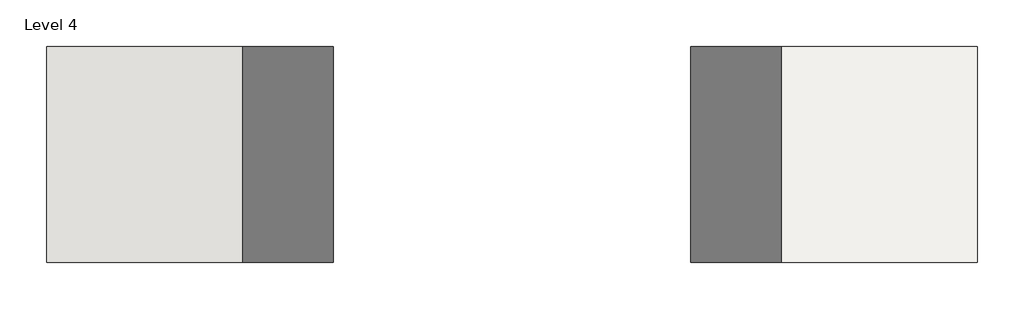
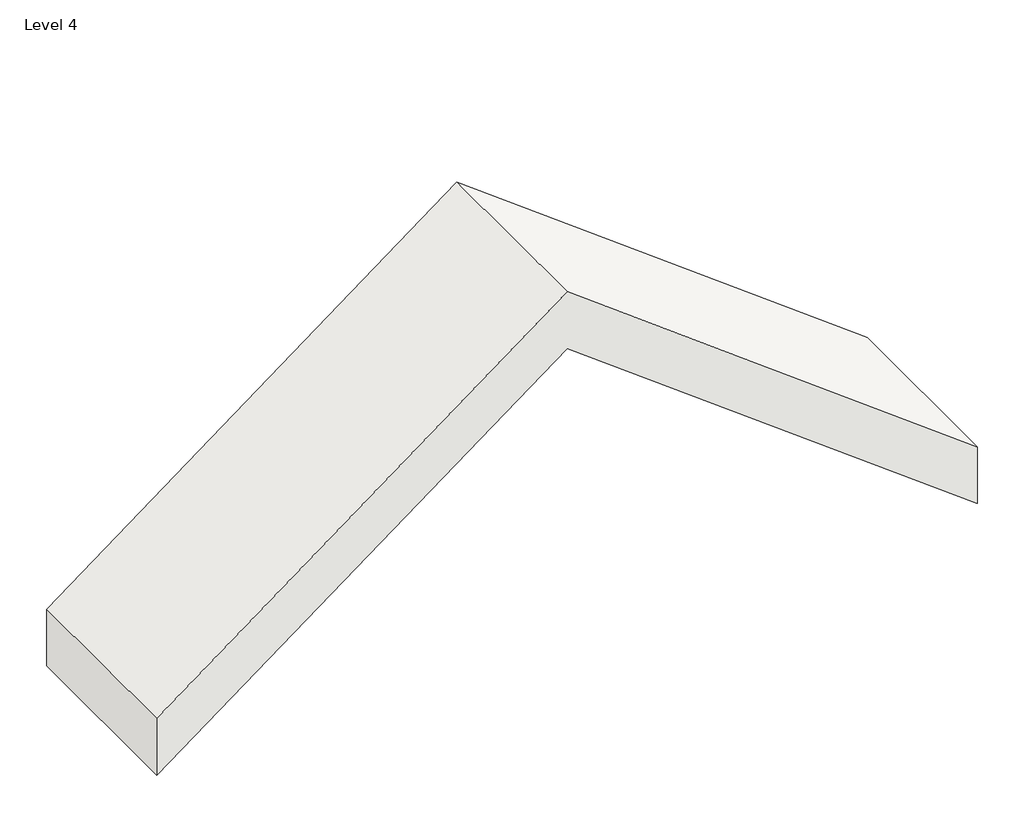
# One storey: 1 roof.
"""IFC4 building model written with IfcOpenShell, lengths in millimetres."""

from ifc_helpers import new_model, si_unit, frame, origin, place, context, project, spatial, polyline, outline, extrude, element, save

model = new_model("IFC4")

# Units and contexts
model_context = context("Model", 3, world=origin())
ifc_project = project(units=[si_unit("LENGTHUNIT", "METRE", prefix="MILLI")], contexts=[model_context])

# Site, building, storey
site = spatial("IfcSite", under=ifc_project)
building = spatial("IfcBuilding", under=site)
storey = spatial("IfcBuildingStorey", under=building, Name="Level 4", Elevation=9144.0)

# Roof
placement = place(None, origin())
element("IfcRoof", 1, ObjectType="Generic - 12\"", at=placement, inside=storey, context=model_context, shape_type="SweptSolid", body=[
    extrude(outline(polyline([(9525.0, -7574.1800533), (11473.1060475, -10171.6547833), (9525.0, -12769.1295133), (9144.0, -12769.1295133), (11092.1060475, -10171.6547833), (9144.0, -7574.1800533), (9525.0, -7574.1800533)])), frame((0.0, -14497.2531473, 0.0), z_axis=(0.0, 1.0, 0.0), x_axis=(0.0, 0.0, 1.0)), (0.0, 0.0, 1.0), 1206.5),
])

save(model, "model.ifc")

# Revit data of these elements
# Type "Generic - 12\""
#   Assembly Code = "B1020"
#   Layers, outside or top first: 1' - 0" no material (function 1)
# Element 1 (IfcRoof, "Generic - 12\"")
#   built-in parameter 1001705 = 37.6414 (stored number, unit not read)
#   built-in parameter 1001710 = 33615
#   Phase Created = New Construction
#   Materials on its faces: "Default Roof"
# Materials
#   "Default Roof": colour RGB 88 101 114, transparency 0, Cost = 0
